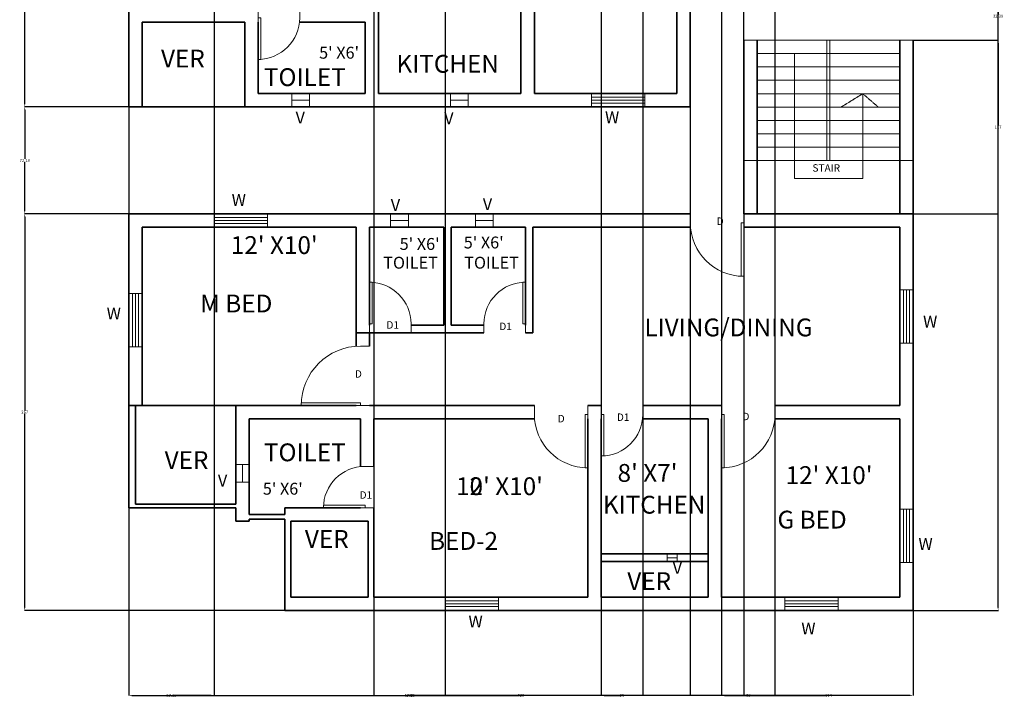
# Model space of a CAD drawing. Units: inches. Extents: x 168 to 831, y 504 to 1681.
# Tile 1 of 3: x 168 to 831, y 504 to 961. Entities that reach past the tile are written whole.
import ezdxf

# ---------------------------------------------------------------- set-up
doc = ezdxf.new("R2010")
doc.units = ezdxf.units.IN
doc.header["$MEASUREMENT"] = 0
doc.linetypes.add('HIDDEN', pattern=[0.375, 0.25, -0.125])
for name, color, linetype, lineweight in [('A-ANNO-DIMS', 2, 'Continuous', 13), ('A-ANNO-TEXT', 7, 'Continuous', 18), ('A-AREA-IDEN', 7, 'Continuous', 18), ('A-DOOR', 3, 'Continuous', 18), ('A-FLOR-STRS', 8, 'Continuous', 18), ('A-FLOR-STRS-PATH', 2, 'HIDDEN', 13), ('A-GLAZ', 4, 'Continuous', 18), ('A-WALL', 7, 'Continuous', 35)]:
    doc.layers.add(name, color=color, linetype=linetype, lineweight=lineweight)
doc.styles.get("Standard").update_dxf_attribs({"font": 'arial.ttf'})
doc.dimstyles.get("Standard").update_dxf_attribs({"dimtxt": 2, "dimasz": 2, "dimexe": 0.18, "dimexo": 0.0625, "dimgap": 0.09, "dimtad": 0, "dimtih": 1, "dimtoh": 1, "dimdec": 0, "dimzin": 0, "dimdsep": 46, "dimlunit": 3, "dimtxsty": 'Standard', "dimcen": 0.09, "dimadec": 0, "dimazin": 0, "dimtfac": 1, "dimtdec": 0, "dimtofl": 0, "dimtmove": 0, "dimatfit": 3, "dimfxl": 1, "dimtolj": 1, "dimtzin": 0, "dimarcsym": 0})

# ---------------------------------------------------------------- blocks, each defined once
blk = doc.blocks.new('*U12')
for p, q in [((-28, 0), (-28, 6)), ((0, 0), (0, 6))]:
    blk.add_line(p, q)
blk.add_lwpolyline([(0, 0), (0, -28), (-1.75, -28), (-1.75, 0)], close=True)
blk.add_arc((0, 0), 28, 180, 270)
blk = doc.blocks.new('*U2')
for p, q in [((0, 0), (0, -6)), ((36, 0), (36, -6))]:
    blk.add_line(p, q)
blk.add_lwpolyline([(0, 0), (0, 36), (1.75, 36), (1.75, 0)], close=True)
blk.add_arc((0, 0), 36, 0, 90)
blk = doc.blocks.new('*U3')
for p, q in [((0, 0), (0, -6)), ((-36, 0), (-36, -6))]:
    blk.add_line(p, q)
blk.add_lwpolyline([(0, 0), (0, 36), (-1.75, 36), (-1.75, 0)], close=True)
blk.add_arc((0, 0), 36, 90, 180)
blk = doc.blocks.new('*U4')
for p, q in [((0, 0), (0, -6)), ((28, 0), (28, -6))]:
    blk.add_line(p, q)
blk.add_lwpolyline([(0, 0), (0, 28), (1.75, 28), (1.75, 0)], close=True)
blk.add_arc((0, 0), 28, 0, 90)
blk = doc.blocks.new('*U5')
for p, q in [((-28, 0), (-28, -6)), ((0, 0), (0, -6))]:
    blk.add_line(p, q)
blk.add_lwpolyline([(0, 0), (0, 28), (-1.75, 28), (-1.75, 0)], close=True)
blk.add_arc((0, 0), 28, 90, 180)
blk = doc.blocks.new('*U6')
for p, q in [((0, 0), (0, -6)), ((28, 0), (28, -6))]:
    blk.add_line(p, q)
blk.add_lwpolyline([(0, 0), (0, 28), (1.75, 28), (1.75, 0)], close=True)
blk.add_arc((0, 0), 28, 0, 90)
blk = doc.blocks.new('*U7')
for p, q in [((0, 0), (0, -6)), ((40, 0), (40, -6))]:
    blk.add_line(p, q)
blk.add_lwpolyline([(0, 0), (0, 40), (1.75, 40), (1.75, 0)], close=True)
blk.add_arc((0, 0), 40, 0, 90)
blk = doc.blocks.new('*U8')
for p, q in [((0, 0), (0, -6)), ((28, 0), (28, -6))]:
    blk.add_line(p, q)
blk.add_lwpolyline([(0, 0), (0, 28), (1.75, 28), (1.75, 0)], close=True)
blk.add_arc((0, 0), 28, 0, 90)
blk = doc.blocks.new('WIN-36IN')
for p, q in [((0, 6.5), (36, 6.5)), ((0, 4.5), (36, 4.5)), ((0, 2.5), (36, 2.5))]:
    blk.add_line(p, q)
blk.add_lwpolyline([(36, 0), (36, 9), (0, 9), (0, 0)], close=True)
blk = doc.blocks.new('VENT-12IN')
blk.add_line((0, 4.5), (12, 4.5))
blk.add_lwpolyline([(0, 0), (0, 9), (12, 9), (12, 0)], close=True)
blk = doc.blocks.new('VENT-KITCHEN-SMALL')
blk.add_line((0, 2.52), (6.62, 2.52))
blk.add_lwpolyline([(0, 0.03), (0, 5), (6.62, 5), (6.62, 0)], close=True)
blk = doc.blocks.new('*D30')
at = {"layer": 'A-ANNO-DIMS', "color": 0, "lineweight": -2, "transparency": 16777216}
for p, q in [((241.86, 631.85), (241.86, 505.48)), ((769.86, 562.85), (769.86, 505.48)), ((243.86, 505.66), (503.56, 505.66)), ((767.86, 505.66), (508.16, 505.66))]:
    blk.add_line(p, q, dxfattribs=at)
at = {"layer": 'A-ANNO-DIMS', "color": 0, "transparency": 16777216}
for points in [[(243.86, 505.99), (243.86, 505.32), (241.86, 505.66)], [(767.86, 505.99), (767.86, 505.32), (769.86, 505.66)]]:
    blk.add_solid(points, dxfattribs=at)
at = {"layer": 'Defpoints', "color": 0, "transparency": 16777216}
for p in [(241.86, 631.91), (769.86, 562.91), (769.86, 505.66)]:
    blk.add_point(p, dxfattribs=at)
at = {"layer": 'A-ANNO-DIMS', "color": 0, "transparency": 16777216, "insert": (505.86, 505.66), "char_height": 2, "attachment_point": 5}
blk.add_mtext('\\A1;528', dxfattribs=at)
blk = doc.blocks.new('*D31')
at = {"layer": 'A-ANNO-DIMS', "color": 0, "lineweight": -2, "transparency": 16777216}
for p, q in [((769.93, 1622.04), (827.29, 1622.04)), ((827.11, 1620.04), (827.11, 1093.58)), ((827.11, 564.91), (827.11, 1091.36)), ((769.93, 562.91), (827.29, 562.91))]:
    blk.add_line(p, q, dxfattribs=at)
at = {"layer": 'A-ANNO-DIMS', "color": 0, "transparency": 16777216}
for points in [[(826.78, 1620.04), (827.45, 1620.04), (827.11, 1622.04)], [(826.78, 564.91), (827.45, 564.91), (827.11, 562.91)]]:
    blk.add_solid(points, dxfattribs=at)
at = {"layer": 'Defpoints', "color": 0, "transparency": 16777216}
for p in [(769.86, 1622.04), (827.11, 1622.04), (769.86, 562.91)]:
    blk.add_point(p, dxfattribs=at)
at = {"layer": 'A-ANNO-DIMS', "color": 0, "transparency": 16777216, "insert": (827.11, 1092.47), "char_height": 2, "attachment_point": 5}
blk.add_mtext('\\A1;1059.1', dxfattribs=at)
blk = doc.blocks.new('*D32')
at = {"layer": 'A-ANNO-DIMS', "color": 0, "lineweight": -2, "transparency": 16777216}
for p, q in [((241.8, 829.91), (171.56, 829.91)), ((171.74, 827.91), (171.74, 697.52)), ((171.74, 564.91), (171.74, 695.3)), ((346.8, 562.91), (171.56, 562.91))]:
    blk.add_line(p, q, dxfattribs=at)
at = {"layer": 'A-ANNO-DIMS', "color": 0, "transparency": 16777216}
for points in [[(171.41, 827.91), (172.08, 827.91), (171.74, 829.91)], [(171.41, 564.91), (172.08, 564.91), (171.74, 562.91)]]:
    blk.add_solid(points, dxfattribs=at)
at = {"layer": 'Defpoints', "color": 0, "transparency": 16777216}
for p in [(171.74, 829.91), (241.86, 829.91), (346.86, 562.91)]:
    blk.add_point(p, dxfattribs=at)
at = {"layer": 'A-ANNO-DIMS', "color": 0, "transparency": 16777216, "insert": (171.74, 696.41), "char_height": 2, "attachment_point": 5}
blk.add_mtext('\\A1;267', dxfattribs=at)
blk = doc.blocks.new('*D33')
at = {"layer": 'A-ANNO-DIMS', "color": 0, "lineweight": -2, "transparency": 16777216}
for p, q in [((241.8, 902.04), (171.56, 902.04)), ((171.74, 900.04), (171.74, 867.09)), ((171.74, 831.91), (171.74, 864.86)), ((241.8, 829.91), (171.56, 829.91))]:
    blk.add_line(p, q, dxfattribs=at)
at = {"layer": 'A-ANNO-DIMS', "color": 0, "transparency": 16777216}
for points in [[(171.41, 900.04), (172.08, 900.04), (171.74, 902.04)], [(171.41, 831.91), (172.08, 831.91), (171.74, 829.91)]]:
    blk.add_solid(points, dxfattribs=at)
at = {"layer": 'Defpoints', "color": 0, "transparency": 16777216}
for p in [(171.74, 902.04), (241.86, 902.04), (241.86, 829.91)]:
    blk.add_point(p, dxfattribs=at)
at = {"layer": 'A-ANNO-DIMS', "color": 0, "transparency": 16777216, "insert": (171.74, 865.97), "char_height": 2, "attachment_point": 5}
blk.add_mtext('\\A1;72.13', dxfattribs=at)
blk = doc.blocks.new('*D34')
at = {"layer": 'A-ANNO-DIMS', "color": 0, "lineweight": -2, "transparency": 16777216}
for p, q in [((241.8, 1283.04), (171.56, 1283.04)), ((171.74, 1281.04), (171.74, 1093.65)), ((171.74, 904.04), (171.74, 1091.43)), ((241.8, 902.04), (171.56, 902.04))]:
    blk.add_line(p, q, dxfattribs=at)
at = {"layer": 'A-ANNO-DIMS', "color": 0, "transparency": 16777216}
for points in [[(171.41, 1281.04), (172.08, 1281.04), (171.74, 1283.04)], [(171.41, 904.04), (172.08, 904.04), (171.74, 902.04)]]:
    blk.add_solid(points, dxfattribs=at)
at = {"layer": 'Defpoints', "color": 0, "transparency": 16777216}
for p in [(171.74, 1283.04), (241.86, 1283.04), (241.86, 902.04)]:
    blk.add_point(p, dxfattribs=at)
at = {"layer": 'A-ANNO-DIMS', "color": 0, "transparency": 16777216, "insert": (171.74, 1092.54), "char_height": 2, "attachment_point": 5}
blk.add_mtext('\\A1;381', dxfattribs=at)
blk = doc.blocks.new('*D39')
at = {"layer": 'A-ANNO-DIMS', "color": 0, "lineweight": -2, "transparency": 16777216}
for p, q in [((241.86, 901.98), (241.86, 505.48)), ((619.86, 901.98), (619.86, 505.48)), ((243.86, 505.66), (428.56, 505.66)), ((617.86, 505.66), (433.16, 505.66))]:
    blk.add_line(p, q, dxfattribs=at)
at = {"layer": 'A-ANNO-DIMS', "color": 0, "transparency": 16777216}
for points in [[(243.86, 505.99), (243.86, 505.32), (241.86, 505.66)], [(617.86, 505.99), (617.86, 505.32), (619.86, 505.66)]]:
    blk.add_solid(points, dxfattribs=at)
at = {"layer": 'Defpoints', "color": 0, "transparency": 16777216}
for p in [(241.86, 902.04), (619.86, 902.04), (619.86, 505.66)]:
    blk.add_point(p, dxfattribs=at)
at = {"layer": 'A-ANNO-DIMS', "color": 0, "transparency": 16777216, "insert": (430.86, 505.66), "char_height": 2, "attachment_point": 5}
blk.add_mtext('\\A1;378', dxfattribs=at)
blk = doc.blocks.new('*D40')
at = {"layer": 'A-ANNO-DIMS', "color": 0, "lineweight": -2, "transparency": 16777216}
for p, q in [((619.86, 902.1), (619.86, 1679.47)), ((621.86, 1679.29), (636.34, 1679.29)), ((653.86, 1679.29), (639.38, 1679.29)), ((655.86, 946.97), (655.86, 1679.47))]:
    blk.add_line(p, q, dxfattribs=at)
at = {"layer": 'A-ANNO-DIMS', "color": 0, "transparency": 16777216}
for points in [[(621.86, 1679.62), (621.86, 1678.96), (619.86, 1679.29)], [(653.86, 1679.62), (653.86, 1678.96), (655.86, 1679.29)]]:
    blk.add_solid(points, dxfattribs=at)
at = {"layer": 'Defpoints', "color": 0, "transparency": 16777216}
for p in [(655.86, 1679.29), (655.86, 946.91), (619.86, 902.04)]:
    blk.add_point(p, dxfattribs=at)
at = {"layer": 'A-ANNO-DIMS', "color": 0, "transparency": 16777216, "insert": (637.86, 1679.29), "char_height": 2, "attachment_point": 5}
blk.add_mtext('\\A1;36', dxfattribs=at)
blk = doc.blocks.new('*D41')
at = {"layer": 'A-ANNO-DIMS', "color": 0, "lineweight": -2, "transparency": 16777216}
for p, q in [((655.86, 829.85), (655.86, 505.48)), ((769.86, 829.85), (769.86, 505.48)), ((657.86, 505.66), (710.66, 505.66)), ((767.86, 505.66), (715.06, 505.66))]:
    blk.add_line(p, q, dxfattribs=at)
at = {"layer": 'A-ANNO-DIMS', "color": 0, "transparency": 16777216}
for points in [[(657.86, 505.99), (657.86, 505.32), (655.86, 505.66)], [(767.86, 505.99), (767.86, 505.32), (769.86, 505.66)]]:
    blk.add_solid(points, dxfattribs=at)
at = {"layer": 'Defpoints', "color": 0, "transparency": 16777216}
for p in [(655.86, 829.91), (769.86, 829.91), (769.86, 505.66)]:
    blk.add_point(p, dxfattribs=at)
at = {"layer": 'A-ANNO-DIMS', "color": 0, "transparency": 16777216, "insert": (712.86, 505.66), "char_height": 2, "attachment_point": 5}
blk.add_mtext('\\A1;114', dxfattribs=at)
blk = doc.blocks.new('*D42')
at = {"layer": 'A-ANNO-DIMS', "color": 0, "lineweight": -2, "transparency": 16777216}
for p, q in [((769.93, 946.91), (827.29, 946.91)), ((827.11, 944.91), (827.11, 889.5)), ((827.11, 831.91), (827.11, 887.31)), ((769.93, 829.91), (827.29, 829.91))]:
    blk.add_line(p, q, dxfattribs=at)
at = {"layer": 'A-ANNO-DIMS', "color": 0, "transparency": 16777216}
for points in [[(826.78, 944.91), (827.45, 944.91), (827.11, 946.91)], [(826.78, 831.91), (827.45, 831.91), (827.11, 829.91)]]:
    blk.add_solid(points, dxfattribs=at)
at = {"layer": 'Defpoints', "color": 0, "transparency": 16777216}
for p in [(769.86, 946.91), (827.11, 946.91), (769.86, 829.91)]:
    blk.add_point(p, dxfattribs=at)
at = {"layer": 'A-ANNO-DIMS', "color": 0, "transparency": 16777216, "insert": (827.11, 888.41), "char_height": 2, "attachment_point": 5}
blk.add_mtext('\\A1;117', dxfattribs=at)
blk = doc.blocks.new('*D43')
at = {"layer": 'A-ANNO-DIMS', "color": 0, "lineweight": -2, "transparency": 16777216}
for p, q in [((769.93, 979.3), (827.29, 979.3)), ((827.11, 977.3), (827.11, 964.22)), ((827.11, 948.91), (827.11, 961.99)), ((769.93, 946.91), (827.29, 946.91))]:
    blk.add_line(p, q, dxfattribs=at)
at = {"layer": 'A-ANNO-DIMS', "color": 0, "transparency": 16777216}
for points in [[(826.78, 977.3), (827.45, 977.3), (827.11, 979.3)], [(826.78, 948.91), (827.45, 948.91), (827.11, 946.91)]]:
    blk.add_solid(points, dxfattribs=at)
at = {"layer": 'Defpoints', "color": 0, "transparency": 16777216}
for p in [(769.86, 979.3), (827.11, 979.3), (769.86, 946.91)]:
    blk.add_point(p, dxfattribs=at)
at = {"layer": 'A-ANNO-DIMS', "color": 0, "transparency": 16777216, "insert": (827.11, 963.1), "char_height": 2, "attachment_point": 5}
blk.add_mtext('\\A1;32.39', dxfattribs=at)
blk = doc.blocks.new('*D47')
at = {"layer": 'A-ANNO-DIMS', "color": 0, "lineweight": -2, "transparency": 16777216}
for p, q in [((559.86, 1483.98), (559.86, 505.48)), ((587.86, 1483.98), (587.86, 505.48)), ((561.86, 505.66), (572.32, 505.66)), ((585.86, 505.66), (575.4, 505.66))]:
    blk.add_line(p, q, dxfattribs=at)
at = {"layer": 'A-ANNO-DIMS', "color": 0, "transparency": 16777216}
for points in [[(561.86, 505.99), (561.86, 505.32), (559.86, 505.66)], [(585.86, 505.99), (585.86, 505.32), (587.86, 505.66)]]:
    blk.add_solid(points, dxfattribs=at)
at = {"layer": 'Defpoints', "color": 0, "transparency": 16777216}
for p in [(559.86, 1484.04), (587.86, 1484.04), (587.86, 505.66)]:
    blk.add_point(p, dxfattribs=at)
at = {"layer": 'A-ANNO-DIMS', "color": 0, "transparency": 16777216, "insert": (573.86, 505.66), "char_height": 2, "attachment_point": 5}
blk.add_mtext('\\A1;28', dxfattribs=at)
blk = doc.blocks.new('*D48')
at = {"layer": 'A-ANNO-DIMS', "color": 0, "lineweight": -2, "transparency": 16777216}
for p, q in [((640.86, 1483.98), (640.86, 505.48)), ((676.86, 1483.98), (676.86, 505.48)), ((642.86, 505.66), (657.34, 505.66)), ((674.86, 505.66), (660.38, 505.66))]:
    blk.add_line(p, q, dxfattribs=at)
at = {"layer": 'A-ANNO-DIMS', "color": 0, "transparency": 16777216}
for points in [[(642.86, 505.99), (642.86, 505.32), (640.86, 505.66)], [(674.86, 505.99), (674.86, 505.32), (676.86, 505.66)]]:
    blk.add_solid(points, dxfattribs=at)
at = {"layer": 'Defpoints', "color": 0, "transparency": 16777216}
for p in [(640.86, 1484.04), (676.86, 1484.04), (676.86, 505.66)]:
    blk.add_point(p, dxfattribs=at)
at = {"layer": 'A-ANNO-DIMS', "color": 0, "transparency": 16777216, "insert": (658.86, 505.66), "char_height": 2, "attachment_point": 5}
blk.add_mtext('\\A1;36', dxfattribs=at)
blk = doc.blocks.new('*D52')
at = {"layer": 'A-ANNO-DIMS', "color": 0, "lineweight": -2, "transparency": 16777216}
for p, q in [((406.86, 1612.98), (406.86, 505.48)), ((454.72, 1612.98), (454.72, 505.48)), ((408.86, 505.66), (427.29, 505.66)), ((452.72, 505.66), (434.3, 505.66))]:
    blk.add_line(p, q, dxfattribs=at)
at = {"layer": 'A-ANNO-DIMS', "color": 0, "transparency": 16777216}
for points in [[(408.86, 505.99), (408.86, 505.32), (406.86, 505.66)], [(452.72, 505.99), (452.72, 505.32), (454.72, 505.66)]]:
    blk.add_solid(points, dxfattribs=at)
at = {"layer": 'Defpoints', "color": 0, "transparency": 16777216}
for p in [(406.86, 1613.04), (454.72, 1613.04), (454.72, 505.66)]:
    blk.add_point(p, dxfattribs=at)
at = {"layer": 'A-ANNO-DIMS', "color": 0, "transparency": 16777216, "insert": (430.79, 505.66), "char_height": 2, "attachment_point": 5}
blk.add_mtext('\\A1;47.86', dxfattribs=at)
blk = doc.blocks.new('*D53')
at = {"layer": 'A-ANNO-DIMS', "color": 0, "lineweight": -2, "transparency": 16777216}
for p, q in [((241.86, 1354.98), (241.86, 505.48)), ((299.21, 1354.98), (299.21, 505.48)), ((243.86, 505.66), (267.07, 505.66)), ((297.21, 505.66), (274.01, 505.66))]:
    blk.add_line(p, q, dxfattribs=at)
at = {"layer": 'A-ANNO-DIMS', "color": 0, "transparency": 16777216}
for points in [[(243.86, 505.99), (243.86, 505.32), (241.86, 505.66)], [(297.21, 505.99), (297.21, 505.32), (299.21, 505.66)]]:
    blk.add_solid(points, dxfattribs=at)
at = {"layer": 'Defpoints', "color": 0, "transparency": 16777216}
for p in [(241.86, 1355.04), (299.21, 1355.04), (299.21, 505.66)]:
    blk.add_point(p, dxfattribs=at)
at = {"layer": 'A-ANNO-DIMS', "color": 0, "transparency": 16777216, "insert": (270.54, 505.66), "char_height": 2, "attachment_point": 5}
blk.add_mtext('\\A1;57.35', dxfattribs=at)

msp = doc.modelspace()

# ---------------------------------------------------------------- linework, layer by layer
at = {"layer": 'A-FLOR-STRS'}
for p, q in [((655.863, 946.908), (769.863, 946.908)), ((711.863, 946.908), (711.863, 865.908)), ((713.863, 946.908), (713.863, 865.908)), ((664.863, 937.908), (760.863, 937.908)), ((664.863, 928.908), (760.863, 928.908)), ((664.863, 919.908), (760.863, 919.908)), ((664.863, 910.908), (760.863, 910.908)), ((664.863, 901.908), (760.863, 901.908)), ((664.863, 892.908), (760.863, 892.908)), ((664.863, 883.908), (760.863, 883.908)), ((664.863, 874.908), (760.863, 874.908)), ((655.863, 865.908), (769.863, 865.908))]:
    msp.add_line(p, q, dxfattribs=at)
at = {"layer": 'A-FLOR-STRS-PATH'}
for p, q in [((690.086, 937.908), (690.086, 865.908)), ((736.018, 910.908), (721.434, 901.908)), ((736.018, 853.741), (736.018, 910.908)), ((746.364, 901.908), (736.018, 910.908)), ((736.018, 910.908), (736.018, 910.908)), ((721.434, 901.908), (746.364, 901.908)), ((690.086, 865.908), (690.086, 865.908)), ((690.086, 865.908), (690.086, 853.741)), ((690.086, 853.741), (736.018, 853.741))]:
    msp.add_line(p, q, dxfattribs=at)
at = {"layer": 'A-WALL'}
for p, q in [((241.863, 902.039), (241.863, 1283.039)), ((514.863, 1004.039), (514.863, 911.039)), ((610.863, 1004.164), (610.863, 911.039)), ((619.863, 1004.039), (619.863, 902.039)), ((409.863, 995.039), (409.863, 911.039)), ((505.863, 995.039), (505.863, 911.039)), ((250.863, 959.039), (319.863, 959.039)), ((250.863, 902.039), (250.863, 959.039)), ((319.863, 959.039), (319.863, 902.039)), ((328.863, 959.039), (328.863, 911.039)), ((356.702, 959.039), (400.863, 959.039)), ((400.863, 959.039), (400.863, 911.039)), ((655.863, 946.908), (655.863, 829.908)), ((664.863, 946.908), (664.863, 829.908)), ((760.863, 946.908), (760.863, 829.908)), ((769.863, 946.908), (769.863, 562.908)), ((328.863, 911.039), (400.863, 911.039)), ((409.863, 911.039), (505.863, 911.039)), ((514.863, 911.039), (610.863, 911.039)), ((241.863, 902.039), (619.863, 902.039)), ((241.863, 776.403), (241.863, 829.908)), ((241.863, 829.908), (241.863, 700.908)), ((241.863, 829.908), (619.863, 829.908)), ((655.863, 829.908), (769.863, 829.908)), ((394.863, 820.908), (250.863, 820.908)), ((250.863, 820.908), (250.863, 700.908)), ((250.863, 820.908), (250.863, 700.908)), ((394.863, 740.796), (394.863, 820.908)), ((453.863, 820.908), (403.863, 820.908)), ((403.863, 754.908), (403.863, 820.908)), ((403.863, 754.908), (403.863, 820.908)), ((453.863, 820.908), (453.863, 754.908)), ((508.863, 820.908), (458.863, 820.908)), ((458.863, 820.908), (458.863, 754.908)), ((458.863, 754.908), (458.863, 820.908)), ((508.863, 820.908), (508.863, 754.908)), ((619.863, 820.908), (513.863, 820.908)), ((513.863, 820.908), (513.863, 749.908)), ((760.863, 820.908), (655.863, 820.908)), ((760.863, 700.908), (760.863, 820.908)), ((458.863, 749.908), (394.863, 749.908)), ((403.863, 740.908), (403.863, 749.908)), ((453.863, 754.908), (431.863, 754.908)), ((480.863, 754.908), (458.863, 754.908)), ((480.863, 749.908), (458.863, 749.908)), ((513.863, 749.908), (508.863, 749.908)), ((241.863, 700.908), (241.863, 631.908)), ((241.863, 700.908), (394.863, 700.908)), ((246.363, 700.908), (246.363, 634.408)), ((250.863, 700.908), (394.863, 700.908)), ((250.863, 700.908), (394.863, 700.908)), ((313.863, 700.908), (313.863, 636.908)), ((403.863, 700.908), (514.863, 700.908)), ((550.863, 700.908), (559.863, 700.908)), ((587.863, 700.908), (640.863, 700.908)), ((676.863, 700.908), (760.863, 700.908)), ((397.863, 691.908), (322.863, 691.908)), ((322.863, 691.908), (322.863, 627.408)), ((397.863, 691.908), (397.863, 659.747)), ((514.989, 691.908), (406.863, 691.908)), ((406.863, 691.908), (406.863, 659.908)), ((550.863, 571.908), (550.863, 691.908)), ((559.863, 571.908), (559.863, 691.908)), ((631.863, 691.908), (587.702, 691.908)), ((631.863, 571.908), (631.863, 691.908)), ((640.863, 571.908), (640.863, 691.908)), ((640.863, 691.908), (640.863, 691.908)), ((760.863, 691.908), (676.863, 691.908)), ((760.863, 571.908), (760.863, 691.908)), ((313.863, 636.908), (313.863, 634.408)), ((313.863, 631.908), (241.863, 631.908)), ((313.863, 634.408), (246.363, 634.408)), ((313.863, 631.908), (313.863, 622.908)), ((397.863, 631.908), (346.863, 631.908)), ((346.863, 627.408), (346.863, 631.908)), ((406.863, 631.908), (406.863, 571.908)), ((346.863, 627.408), (322.863, 627.408)), ((322.863, 624.408), (322.863, 622.908)), ((346.863, 624.408), (322.863, 624.408)), ((346.863, 627.408), (346.863, 627.408)), ((346.863, 622.908), (346.863, 624.408)), ((322.863, 622.908), (313.863, 622.908)), ((346.863, 622.908), (346.863, 562.908)), ((402.863, 622.908), (350.863, 622.908)), ((350.863, 622.908), (350.863, 571.908)), ((402.863, 622.908), (402.863, 571.908)), ((559.863, 602.908), (559.863, 571.908)), ((631.863, 600.908), (559.863, 600.908)), ((631.863, 595.908), (559.863, 595.908)), ((350.863, 571.908), (402.863, 571.908)), ((406.863, 571.908), (550.863, 571.908)), ((559.863, 571.908), (631.863, 571.908)), ((640.863, 571.908), (760.863, 571.908)), ((346.863, 562.908), (769.863, 562.908))]:
    msp.add_line(p, q, dxfattribs=at)

# ---------------------------------------------------------------- block references
at = {"layer": 'A-DOOR', "xscale": -1}
msp.add_blockref('*U12', (328.863, 962.039), dxfattribs=at)
at = {"layer": 'A-DOOR', "xscale": -1, "rotation": 180}
for name, p in [('*U3', (655.863, 823.908)), ('*U4', (559.863, 694.908)), ('*U2', (640.863, 694.908))]:
    msp.add_blockref(name, p, dxfattribs=at)
at = {"layer": 'A-DOOR'}
for name, p in [('*U6', (403.863, 755.908)), ('*U5', (508.863, 755.908))]:
    msp.add_blockref(name, p, dxfattribs=at)
for name, p, rotation in [('*U7', (397.863, 700.908), 90.00000000000003), ('*U2', (550.863, 694.908), 180), ('*U8', (400.863, 631.908), 90.00000000000003)]:
    msp.add_blockref(name, p, dxfattribs=dict(at, rotation=rotation))
at = {"layer": 'A-GLAZ'}
for name, p in [('VENT-12IN', (351.526, 901.978)), ('VENT-12IN', (458.341, 902.039)), ('WIN-36IN', (553.319, 902.039)), ('WIN-36IN', (553.319, 902.039))]:
    msp.add_blockref(name, p, dxfattribs=at)
at = {"layer": 'A-GLAZ', "extrusion": (0, 0, -1), "zscale": -1}
for name, p, rotation in [('WIN-36IN', (-299.212, 829.908), 180), ('WIN-36IN', (-299.212, 829.908), 180), ('VENT-12IN', (-418.112, 829.908), 180), ('VENT-12IN', (-475.211, 829.908), 180), ('WIN-36IN', (-241.864, 740.403), 90.00000000000087), ('WIN-36IN', (-760.864, 742.835), 90.00000000000102), ('VENT-12IN', (-322.863, 661.253), 269.9999999999985), ('WIN-36IN', (-760.864, 595.098), 90.00000000000078), ('VENT-KITCHEN-SMALL', (-604.305, 600.908), 180), ('WIN-36IN', (-454.72, 571.908), 180), ('WIN-36IN', (-683.502, 571.908), 180)]:
    msp.add_blockref(name, p, dxfattribs=dict(at, rotation=rotation))

# ---------------------------------------------------------------- texts
at = {"layer": 'A-ANNO-DIMS', "attachment_point": 1}
for s, width, insert, char_height in [("5' X6'", 59.10581, (369.961, 942.507), 8), ("12' X10'", 157.93148, (310.488, 814.934), 12), ("5' X6'", 59.10581, (424.188, 813.697), 8), ("5' X6'", 59.10581, (467.327, 814.673), 8), ("8' X7'", 157.93148, (570.883, 661.481), 12), ("12' X10'", 157.93148, (684.045, 660.007), 12), ("12' X10'", 157.93148, (462.133, 652.545), 12), ("10' X10'", 157.93148, (462.133, 652.545), 12), ("5' X6'", 59.10581, (332.054, 648.836), 8)]:
    msp.add_mtext_dynamic_manual_height_columns(s, width=width, gutter_width=1, heights=[0], dxfattribs=dict(at, insert=insert, char_height=char_height))
at = {"layer": 'A-ANNO-TEXT'}
for s, width, insert, char_height, attachment_point in [('V', 20.00841, (354.103, 898.9), 8, 1), ('V', 20.00841, (454.172, 898.376), 8, 1), ('W', 57.92772, (562.437, 899.048), 8, 1), ('W', 57.92772, (311.064, 843.31), 8, 1), ('V', 20.00841, (418.174, 839.917), 8, 1), ('V', 20.00841, (480.171, 840.536), 8, 1), ('D', 11.24528, (637.616, 822.564), 5, 7), ('W', 57.92772, (226.906, 766.852), 8, 1), ('D1', 11.24528, (415.277, 752.644), 5, 7), ('D1', 11.24528, (491.256, 751.712), 5, 7), ('W', 57.92772, (776.589, 761.392), 8, 1), ('D', 11.24528, (394.021, 719.636), 5, 7), ('D', 11.24528, (530.576, 689.542), 5, 7), ('D1', 11.24528, (570.425, 690.513), 5, 7), ('D', 11.24528, (654.982, 690.998), 5, 7), ('V', 20.00841, (301.799, 654.302), 8, 1), ('D1', 11.24528, (397.209, 638.108), 5, 7), ('W', 57.92772, (773.466, 611.654), 8, 1), ('V', 20.00841, (608.008, 595.519), 8, 1), ('W', 57.92772, (470.516, 559.402), 8, 1), ('W', 57.92772, (694.605, 554.723), 8, 1)]:
    msp.add_mtext_dynamic_manual_height_columns(s, width=width, gutter_width=1, heights=[0], dxfattribs=dict(at, insert=insert, char_height=char_height, attachment_point=attachment_point))
at = {"layer": 'A-AREA-IDEN'}
for s, width, insert, char_height, attachment_point in [('VER', 54.54242, (263.513, 940.559), 12, 1), ('KITCHEN', 54.54242, (422.004, 937.018), 12, 1), ('TOILET', 54.54242, (332.756, 928.038), 12, 1), ('STAIR', 11.78067, (702.083, 863.4), 5, 1), ('TOILET', 54.54242, (413.129, 793.061), 8, 7), ('TOILET', 54.54242, (467.672, 793.061), 8, 7), ('M BED', 54.54242, (289.837, 763.585), 12, 7), ('LIVING/DINING', 54.54242, (588.938, 747.473), 12, 7), ('VER', 54.54242, (265.944, 658.09), 12, 7), ('TOILET', 54.54242, (332.756, 663.341), 12, 7), ('KITCHEN', 54.54242, (561.014, 628.058), 12, 7), ('G BED', 54.54242, (678.553, 618.027), 12, 7), ('VER', 54.54242, (360.361, 605.024), 12, 7), ('BED-2', 54.54242, (443.993, 603.674), 12, 7), ('VER', 54.54242, (577.442, 576.58), 12, 7)]:
    msp.add_mtext_dynamic_manual_height_columns(s, width=width, gutter_width=1, heights=[0], dxfattribs=dict(at, insert=insert, char_height=char_height, attachment_point=attachment_point))

# ---------------------------------------------------------------- dimensions: what is measured, and where the dimension line sits
at = {"layer": 'A-ANNO-DIMS'}
for base, p1, p2, override, picture, middle in [((655.863, 1679.289), (619.863, 902.039), (655.863, 946.908), {"dimdec": 0, "dimlfac": 1, "dimrnd": 0, "dimzin": 0, "dimdsep": 46, "dimlunit": 2}, '*D40', (637.863, 1679.289)), ((454.72, 505.658), (406.863, 1613.039), (454.72, 1613.039), {"dimdec": 2, "dimlfac": 1, "dimrnd": 0, "dimzin": 0, "dimdsep": 46, "dimlunit": 2}, '*D52', (430.792, 505.658)), ((587.863, 505.658), (559.863, 1484.039), (587.863, 1484.039), {"dimdec": 0, "dimlfac": 1, "dimrnd": 0, "dimzin": 0, "dimdsep": 46, "dimlunit": 2}, '*D47', (573.863, 505.658)), ((676.863, 505.658), (640.863, 1484.039), (676.863, 1484.039), {"dimdec": 0, "dimlfac": 1, "dimrnd": 0, "dimzin": 0, "dimdsep": 46, "dimlunit": 2}, '*D48', (658.863, 505.658)), ((299.213, 505.658), (241.863, 1355.039), (299.213, 1355.039), {"dimdec": 2, "dimlfac": 1, "dimrnd": 0, "dimzin": 0, "dimdsep": 46, "dimlunit": 2}, '*D53', (270.538, 505.658)), ((619.863, 505.658), (241.863, 902.039), (619.863, 902.039), {"dimdec": 0, "dimlfac": 1, "dimrnd": 0, "dimzin": 0, "dimdsep": 46, "dimlunit": 2}, '*D39', (430.863, 505.658)), ((769.863, 505.658), (655.863, 829.908), (769.863, 829.908), {"dimdec": 0, "dimlfac": 1, "dimrnd": 0, "dimzin": 0, "dimdsep": 46, "dimlunit": 2}, '*D41', (712.863, 505.658)), ((769.863, 505.658), (241.863, 631.908), (769.863, 562.908), {"dimdec": 0, "dimlfac": 1, "dimrnd": 0, "dimzin": 0, "dimdsep": 46, "dimlunit": 2}, '*D30', (505.863, 505.658))]:
    dim = msp.add_linear_dim(base=base, p1=p1, p2=p2, dimstyle='Standard', override=override, dxfattribs=at)
    dim.commit()
    dim.dimension.update_dxf_attribs({"geometry": picture, "text_midpoint": middle})
for base, p1, p2, override, picture, middle in [((827.113, 1622.039), (769.863, 562.908), (769.863, 1622.039), {"dimdec": 1, "dimlfac": 1, "dimrnd": 0, "dimzin": 0, "dimdsep": 46, "dimlunit": 2}, '*D31', (827.113, 1092.474)), ((171.744, 1283.039), (241.863, 902.039), (241.863, 1283.039), {"dimdec": 0, "dimlfac": 1, "dimrnd": 0, "dimzin": 0, "dimdsep": 46, "dimlunit": 2}, '*D34', (171.744, 1092.539)), ((827.113, 979.3), (769.863, 946.908), (769.863, 979.3), {"dimdec": 2, "dimlfac": 1, "dimrnd": 0, "dimzin": 0, "dimdsep": 46, "dimlunit": 2}, '*D43', (827.113, 963.104)), ((827.113, 946.908), (769.863, 829.908), (769.863, 946.908), {"dimdec": 0, "dimlfac": 1, "dimrnd": 0, "dimzin": 0, "dimdsep": 46, "dimlunit": 2}, '*D42', (827.113, 888.408)), ((171.744, 902.039), (241.863, 829.908), (241.863, 902.039), {"dimdec": 2, "dimlfac": 1, "dimrnd": 0, "dimzin": 0, "dimdsep": 46, "dimlunit": 2}, '*D33', (171.744, 865.974)), ((171.744, 829.908), (346.863, 562.908), (241.863, 829.908), {"dimdec": 0, "dimlfac": 1, "dimrnd": 0, "dimzin": 0, "dimdsep": 46, "dimlunit": 2}, '*D32', (171.744, 696.408))]:
    dim = msp.add_linear_dim(base=base, p1=p1, p2=p2, angle=90, dimstyle='Standard', override=override, dxfattribs=at)
    dim.commit()
    dim.dimension.update_dxf_attribs({"geometry": picture, "text_midpoint": middle})

doc.saveas('drawing.dxf')
